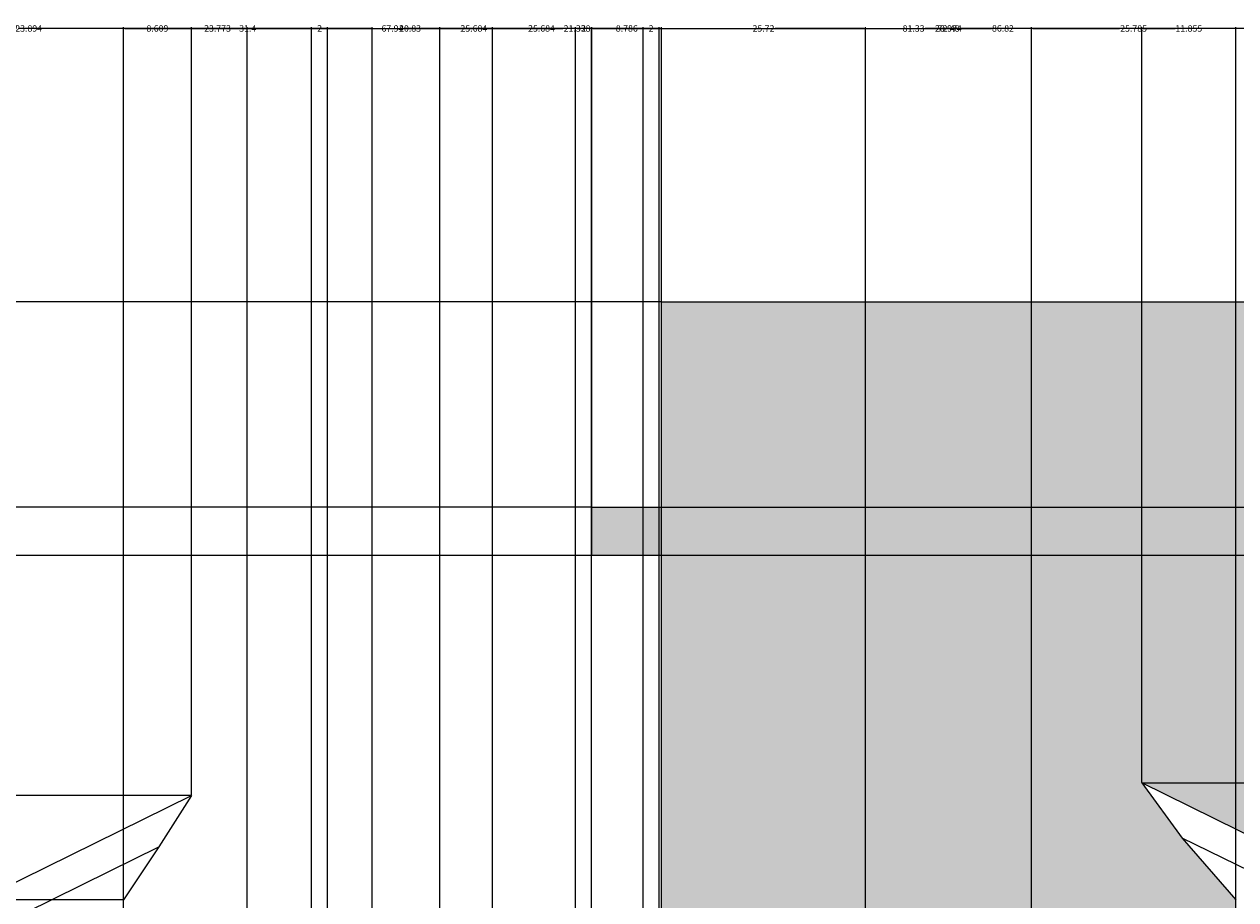
# Model space of a CAD drawing. Units: inches. Extents: x 36 to 594, y 79 to 831.
# Tile 24 of 30: x 189 to 342, y 721 to 831. Entities that reach past the tile are written whole.
import ezdxf

# ---------------------------------------------------------------- set-up
doc = ezdxf.new("R2010")
doc.units = ezdxf.units.IN
doc.header["$MEASUREMENT"] = 0
for name, color, linetype, lineweight in [('A-ANNO-DIMS', 2, 'Continuous', 18), ('A-ELEV', 7, 'Continuous', 25), ('A-ELEV-PATT', 8, 'Continuous', 13)]:
    doc.layers.add(name, color=color, linetype=linetype, lineweight=lineweight)
doc.styles.get("Standard").update_dxf_attribs({"font": 'arial.ttf'})
doc.dimstyles.get("Standard").update_dxf_attribs({"dimtxt": 0.8125, "dimasz": 0.18, "dimexe": 0.18, "dimexo": 0.0625, "dimgap": 0.09, "dimtad": 0, "dimtih": 1, "dimtoh": 1, "dimdec": 4, "dimzin": 0, "dimdsep": 46, "dimlunit": 4, "dimtxsty": 'Standard', "dimcen": 0.09, "dimadec": 0, "dimazin": 0, "dimtfac": 1, "dimtdec": 4, "dimtofl": 0, "dimtmove": 0, "dimatfit": 3, "dimfxl": 1, "dimtolj": 1, "dimtzin": 0, "dimarcsym": 0})

# ---------------------------------------------------------------- blocks, each defined once
blk = doc.blocks.new('*D14')
at = {"layer": 'A-ANNO-DIMS', "color": 0, "lineweight": -2, "transparency": 16777216}
for p, q in [((177.52, 594.27), (177.52, 830.73)), ((177.7, 830.55), (187.69, 830.55)), ((201.24, 830.55), (191.25, 830.55)), ((201.42, 720.66), (201.42, 830.73))]:
    blk.add_line(p, q, dxfattribs=at)
at = {"layer": 'A-ANNO-DIMS', "color": 0, "transparency": 16777216}
for points in [[(177.7, 830.58), (177.7, 830.52), (177.52, 830.55)], [(201.24, 830.58), (201.24, 830.52), (201.42, 830.55)]]:
    blk.add_solid(points, dxfattribs=at)
at = {"layer": 'Defpoints', "color": 0, "transparency": 16777216}
for p in [(201.42, 830.55), (201.42, 720.59), (177.52, 594.21)]:
    blk.add_point(p, dxfattribs=at)
at = {"layer": 'A-ANNO-DIMS', "color": 0, "transparency": 16777216, "insert": (189.47, 830.55), "char_height": 0.812, "attachment_point": 5}
blk.add_mtext('\\A1;23.894', dxfattribs=at)
blk = doc.blocks.new('*D15')
at = {"layer": 'A-ANNO-DIMS', "color": 0, "lineweight": -2, "transparency": 16777216}
for p, q in [((201.42, 720.66), (201.42, 830.73)), ((201.6, 830.55), (233.93, 830.55)), ((269.18, 830.55), (236.85, 830.55)), ((269.36, 796.11), (269.36, 830.73))]:
    blk.add_line(p, q, dxfattribs=at)
at = {"layer": 'A-ANNO-DIMS', "color": 0, "transparency": 16777216}
for points in [[(201.6, 830.58), (201.6, 830.52), (201.42, 830.55)], [(269.18, 830.58), (269.18, 830.52), (269.36, 830.55)]]:
    blk.add_solid(points, dxfattribs=at)
at = {"layer": 'Defpoints', "color": 0, "transparency": 16777216}
for p in [(269.36, 830.55), (269.36, 796.05), (201.42, 720.59)]:
    blk.add_point(p, dxfattribs=at)
at = {"layer": 'A-ANNO-DIMS', "color": 0, "transparency": 16777216, "insert": (235.39, 830.55), "char_height": 0.812, "attachment_point": 5}
blk.add_mtext('\\A1;67.94', dxfattribs=at)
blk = doc.blocks.new('*D16')
at = {"layer": 'A-ANNO-DIMS', "color": 0, "lineweight": -2, "transparency": 16777216}
for p, q in [((269.36, 796.11), (269.36, 830.73)), ((269.54, 830.55), (304.14, 830.55)), ((341.66, 830.55), (307.06, 830.55)), ((341.84, 720.66), (341.84, 830.73))]:
    blk.add_line(p, q, dxfattribs=at)
at = {"layer": 'A-ANNO-DIMS', "color": 0, "transparency": 16777216}
for points in [[(269.54, 830.58), (269.54, 830.52), (269.36, 830.55)], [(341.66, 830.58), (341.66, 830.52), (341.84, 830.55)]]:
    blk.add_solid(points, dxfattribs=at)
at = {"layer": 'Defpoints', "color": 0, "transparency": 16777216}
for p in [(341.84, 830.55), (269.36, 796.05), (341.84, 720.59)]:
    blk.add_point(p, dxfattribs=at)
at = {"layer": 'A-ANNO-DIMS', "color": 0, "transparency": 16777216, "insert": (305.6, 830.55), "char_height": 0.812, "attachment_point": 5}
blk.add_mtext('\\A1;72.48', dxfattribs=at)
blk = doc.blocks.new('*D22')
at = {"layer": 'A-ANNO-DIMS', "color": 0, "lineweight": -2, "transparency": 16777216}
for p, q in [((201.42, 720.66), (201.42, 830.73)), ((201.6, 830.55), (204.26, 830.55)), ((209.85, 830.55), (207.19, 830.55)), ((210.03, 733.8), (210.03, 830.73))]:
    blk.add_line(p, q, dxfattribs=at)
at = {"layer": 'A-ANNO-DIMS', "color": 0, "transparency": 16777216}
for points in [[(201.6, 830.58), (201.6, 830.52), (201.42, 830.55)], [(209.85, 830.58), (209.85, 830.52), (210.03, 830.55)]]:
    blk.add_solid(points, dxfattribs=at)
at = {"layer": 'Defpoints', "color": 0, "transparency": 16777216}
for p in [(210.03, 830.55), (210.03, 733.74), (201.42, 720.59)]:
    blk.add_point(p, dxfattribs=at)
at = {"layer": 'A-ANNO-DIMS', "color": 0, "transparency": 16777216, "insert": (205.72, 830.55), "char_height": 0.812, "attachment_point": 5}
blk.add_mtext('\\A1;8.609', dxfattribs=at)
blk = doc.blocks.new('*D23')
at = {"layer": 'A-ANNO-DIMS', "color": 0, "lineweight": -2, "transparency": 16777216}
for p, q in [((329.98, 735.4), (329.98, 830.73)), ((330.16, 830.55), (334.17, 830.55)), ((341.66, 830.55), (337.65, 830.55)), ((341.84, 720.66), (341.84, 830.73))]:
    blk.add_line(p, q, dxfattribs=at)
at = {"layer": 'A-ANNO-DIMS', "color": 0, "transparency": 16777216}
for points in [[(330.16, 830.58), (330.16, 830.52), (329.98, 830.55)], [(341.66, 830.58), (341.66, 830.52), (341.84, 830.55)]]:
    blk.add_solid(points, dxfattribs=at)
at = {"layer": 'Defpoints', "color": 0, "transparency": 16777216}
for p in [(341.84, 830.55), (329.98, 735.34), (341.84, 720.59)]:
    blk.add_point(p, dxfattribs=at)
at = {"layer": 'A-ANNO-DIMS', "color": 0, "transparency": 16777216, "insert": (335.91, 830.55), "char_height": 0.812, "attachment_point": 5}
blk.add_mtext('\\A1;11.855', dxfattribs=at)
blk = doc.blocks.new('*D25')
at = {"layer": 'A-ANNO-DIMS', "color": 0, "lineweight": -2, "transparency": 16777216}
for p, q in [((260.57, 764.1), (260.57, 830.73)), ((260.75, 830.55), (263.5, 830.55)), ((269.18, 830.55), (266.43, 830.55)), ((269.36, 796.11), (269.36, 830.73))]:
    blk.add_line(p, q, dxfattribs=at)
at = {"layer": 'A-ANNO-DIMS', "color": 0, "transparency": 16777216}
for points in [[(260.75, 830.58), (260.75, 830.52), (260.57, 830.55)], [(269.18, 830.58), (269.18, 830.52), (269.36, 830.55)]]:
    blk.add_solid(points, dxfattribs=at)
at = {"layer": 'Defpoints', "color": 0, "transparency": 16777216}
for p in [(269.36, 830.55), (269.36, 796.05), (260.57, 764.03)]:
    blk.add_point(p, dxfattribs=at)
at = {"layer": 'A-ANNO-DIMS', "color": 0, "transparency": 16777216, "insert": (264.97, 830.55), "char_height": 0.812, "attachment_point": 5}
blk.add_mtext('\\A1;8.786', dxfattribs=at)
blk = doc.blocks.new('*D28')
at = {"layer": 'A-ANNO-DIMS', "color": 0, "lineweight": -2, "transparency": 16777216}
for p, q in [((269.3, 796.05), (37.49, 796.05)), ((37.67, 795.87), (37.67, 455.63)), ((37.67, 114.39), (37.67, 454.62)), ((94.8, 114.21), (37.49, 114.21))]:
    blk.add_line(p, q, dxfattribs=at)
at = {"layer": 'A-ANNO-DIMS', "color": 0, "transparency": 16777216}
for points in [[(37.64, 795.87), (37.7, 795.87), (37.67, 796.05)], [(37.64, 114.39), (37.7, 114.39), (37.67, 114.21)]]:
    blk.add_solid(points, dxfattribs=at)
at = {"layer": 'Defpoints', "color": 0, "transparency": 16777216}
for p in [(37.67, 796.05), (269.36, 796.05), (94.87, 114.21)]:
    blk.add_point(p, dxfattribs=at)
at = {"layer": 'A-ANNO-DIMS', "color": 0, "transparency": 16777216, "insert": (37.67, 455.13), "char_height": 0.812, "attachment_point": 5}
blk.add_mtext('\\A1;681.8', dxfattribs=at)
blk = doc.blocks.new('*D37')
at = {"layer": 'A-ANNO-DIMS', "color": 0, "lineweight": -2, "transparency": 16777216}
for p, q in [((330.04, 735.34), (592.85, 735.34)), ((592.67, 735.16), (592.67, 702.28)), ((592.67, 668.39), (592.67, 701.27)), ((448.45, 668.21), (592.85, 668.21))]:
    blk.add_line(p, q, dxfattribs=at)
at = {"layer": 'A-ANNO-DIMS', "color": 0, "transparency": 16777216}
for points in [[(592.64, 735.16), (592.7, 735.16), (592.67, 735.34)], [(592.64, 668.39), (592.7, 668.39), (592.67, 668.21)]]:
    blk.add_solid(points, dxfattribs=at)
at = {"layer": 'Defpoints', "color": 0, "transparency": 16777216}
for p in [(329.98, 735.34), (592.67, 735.34), (448.39, 668.21)]:
    blk.add_point(p, dxfattribs=at)
at = {"layer": 'A-ANNO-DIMS', "color": 0, "transparency": 16777216, "insert": (592.67, 701.77), "char_height": 0.812, "attachment_point": 5}
blk.add_mtext('\\A1;67.12', dxfattribs=at)
blk = doc.blocks.new('*D38')
at = {"layer": 'A-ANNO-DIMS', "color": 0, "lineweight": -2, "transparency": 16777216}
for p, q in [((398.15, 796.05), (592.85, 796.05)), ((592.67, 795.87), (592.67, 766.2)), ((592.67, 735.52), (592.67, 765.19)), ((330.04, 735.34), (592.85, 735.34))]:
    blk.add_line(p, q, dxfattribs=at)
at = {"layer": 'A-ANNO-DIMS', "color": 0, "transparency": 16777216}
for points in [[(592.64, 795.87), (592.7, 795.87), (592.67, 796.05)], [(592.64, 735.52), (592.7, 735.52), (592.67, 735.34)]]:
    blk.add_solid(points, dxfattribs=at)
at = {"layer": 'Defpoints', "color": 0, "transparency": 16777216}
for p in [(398.09, 796.05), (592.67, 796.05), (329.98, 735.34)]:
    blk.add_point(p, dxfattribs=at)
at = {"layer": 'A-ANNO-DIMS', "color": 0, "transparency": 16777216, "insert": (592.67, 765.69), "char_height": 0.812, "attachment_point": 5}
blk.add_mtext('\\A1;60.71', dxfattribs=at)
blk = doc.blocks.new('*D48')
at = {"layer": 'A-ANNO-DIMS', "color": 0, "lineweight": -2, "transparency": 16777216}
for p, q in [((201.36, 720.59), (37.49, 720.59)), ((37.67, 720.41), (37.67, 694.91)), ((37.67, 668.39), (37.67, 693.9)), ((94.8, 668.21), (37.49, 668.21))]:
    blk.add_line(p, q, dxfattribs=at)
at = {"layer": 'A-ANNO-DIMS', "color": 0, "transparency": 16777216}
for points in [[(37.64, 720.41), (37.7, 720.41), (37.67, 720.59)], [(37.64, 668.39), (37.7, 668.39), (37.67, 668.21)]]:
    blk.add_solid(points, dxfattribs=at)
at = {"layer": 'Defpoints', "color": 0, "transparency": 16777216}
for p in [(37.67, 720.59), (201.42, 720.59), (94.87, 668.21)]:
    blk.add_point(p, dxfattribs=at)
at = {"layer": 'A-ANNO-DIMS', "color": 0, "transparency": 16777216, "insert": (37.67, 694.4), "char_height": 0.812, "attachment_point": 5}
blk.add_mtext('\\A1;52.38', dxfattribs=at)
blk = doc.blocks.new('*D49')
at = {"layer": 'A-ANNO-DIMS', "color": 0, "lineweight": -2, "transparency": 16777216}
for p, q in [((209.97, 733.74), (37.49, 733.74)), ((37.67, 733.56), (37.67, 727.67)), ((37.67, 720.77), (37.67, 726.66)), ((201.36, 720.59), (37.49, 720.59))]:
    blk.add_line(p, q, dxfattribs=at)
at = {"layer": 'A-ANNO-DIMS', "color": 0, "transparency": 16777216}
for points in [[(37.64, 733.56), (37.7, 733.56), (37.67, 733.74)], [(37.64, 720.77), (37.7, 720.77), (37.67, 720.59)]]:
    blk.add_solid(points, dxfattribs=at)
at = {"layer": 'Defpoints', "color": 0, "transparency": 16777216}
for p in [(37.67, 733.74), (210.03, 733.74), (201.42, 720.59)]:
    blk.add_point(p, dxfattribs=at)
at = {"layer": 'A-ANNO-DIMS', "color": 0, "transparency": 16777216, "insert": (37.67, 727.17), "char_height": 0.812, "attachment_point": 5}
blk.add_mtext('\\A1;13.147', dxfattribs=at)
blk = doc.blocks.new('*D50')
at = {"layer": 'A-ANNO-DIMS', "color": 0, "lineweight": -2, "transparency": 16777216}
for p, q in [((260.51, 764.03), (37.49, 764.03)), ((37.67, 763.85), (37.67, 749.39)), ((37.67, 733.92), (37.67, 748.38)), ((209.97, 733.74), (37.49, 733.74))]:
    blk.add_line(p, q, dxfattribs=at)
at = {"layer": 'A-ANNO-DIMS', "color": 0, "transparency": 16777216}
for points in [[(37.64, 763.85), (37.7, 763.85), (37.67, 764.03)], [(37.64, 733.92), (37.7, 733.92), (37.67, 733.74)]]:
    blk.add_solid(points, dxfattribs=at)
at = {"layer": 'Defpoints', "color": 0, "transparency": 16777216}
for p in [(37.67, 764.03), (260.57, 764.03), (210.03, 733.74)]:
    blk.add_point(p, dxfattribs=at)
at = {"layer": 'A-ANNO-DIMS', "color": 0, "transparency": 16777216, "insert": (37.67, 748.89), "char_height": 0.812, "attachment_point": 5}
blk.add_mtext('\\A1;30.29', dxfattribs=at)
blk = doc.blocks.new('*D51')
at = {"layer": 'A-ANNO-DIMS', "color": 0, "lineweight": -2, "transparency": 16777216}
for p, q in [((260.51, 770.15), (37.49, 770.15)), ((37.67, 769.97), (37.67, 767.59)), ((37.67, 764.21), (37.67, 766.58)), ((260.51, 764.03), (37.49, 764.03))]:
    blk.add_line(p, q, dxfattribs=at)
at = {"layer": 'A-ANNO-DIMS', "color": 0, "transparency": 16777216}
for points in [[(37.64, 769.97), (37.7, 769.97), (37.67, 770.15)], [(37.64, 764.21), (37.7, 764.21), (37.67, 764.03)]]:
    blk.add_solid(points, dxfattribs=at)
at = {"layer": 'Defpoints', "color": 0, "transparency": 16777216}
for p in [(37.67, 770.15), (260.57, 770.15), (260.57, 764.03)]:
    blk.add_point(p, dxfattribs=at)
at = {"layer": 'A-ANNO-DIMS', "color": 0, "transparency": 16777216, "insert": (37.67, 767.09), "char_height": 0.812, "attachment_point": 5}
blk.add_mtext('\\A1;6.111', dxfattribs=at)
blk = doc.blocks.new('*D52')
at = {"layer": 'A-ANNO-DIMS', "color": 0, "lineweight": -2, "transparency": 16777216}
for p, q in [((269.3, 796.05), (37.49, 796.05)), ((37.67, 795.87), (37.67, 783.6)), ((37.67, 770.33), (37.67, 782.59)), ((260.51, 770.15), (37.49, 770.15))]:
    blk.add_line(p, q, dxfattribs=at)
at = {"layer": 'A-ANNO-DIMS', "color": 0, "transparency": 16777216}
for points in [[(37.64, 795.87), (37.7, 795.87), (37.67, 796.05)], [(37.64, 770.33), (37.7, 770.33), (37.67, 770.15)]]:
    blk.add_solid(points, dxfattribs=at)
at = {"layer": 'Defpoints', "color": 0, "transparency": 16777216}
for p in [(37.67, 796.05), (269.36, 796.05), (260.57, 770.15)]:
    blk.add_point(p, dxfattribs=at)
at = {"layer": 'A-ANNO-DIMS', "color": 0, "transparency": 16777216, "insert": (37.67, 783.1), "char_height": 0.812, "attachment_point": 5}
blk.add_mtext('\\A1;25.9', dxfattribs=at)
blk = doc.blocks.new('*D61')
at = {"layer": 'A-ANNO-DIMS', "color": 0, "lineweight": -2, "transparency": 16777216}
for p, q in [((156.41, 264.68), (156.41, 830.73)), ((156.59, 830.55), (185.26, 830.55)), ((216.85, 830.55), (188.18, 830.55)), ((217.03, 286.24), (217.03, 830.73))]:
    blk.add_line(p, q, dxfattribs=at)
at = {"layer": 'A-ANNO-DIMS', "color": 0, "transparency": 16777216}
for points in [[(156.59, 830.58), (156.59, 830.52), (156.41, 830.55)], [(216.85, 830.58), (216.85, 830.52), (217.03, 830.55)]]:
    blk.add_solid(points, dxfattribs=at)
at = {"layer": 'Defpoints', "color": 0, "transparency": 16777216}
for p in [(217.03, 830.55), (217.03, 286.18), (156.41, 264.62)]:
    blk.add_point(p, dxfattribs=at)
at = {"layer": 'A-ANNO-DIMS', "color": 0, "transparency": 16777216, "insert": (186.72, 830.55), "char_height": 0.812, "attachment_point": 5}
blk.add_mtext('\\A1;60.62', dxfattribs=at)
blk = doc.blocks.new('*D92')
at = {"layer": 'A-ANNO-DIMS', "color": 0, "lineweight": -2, "transparency": 16777216}
for p, q in [((201.42, 475.48), (201.42, 830.73)), ((201.6, 830.55), (215.98, 830.55)), ((232.64, 830.55), (218.26, 830.55)), ((232.82, 524.67), (232.82, 830.73))]:
    blk.add_line(p, q, dxfattribs=at)
at = {"layer": 'A-ANNO-DIMS', "color": 0, "transparency": 16777216}
for points in [[(201.6, 830.58), (201.6, 830.52), (201.42, 830.55)], [(232.64, 830.58), (232.64, 830.52), (232.82, 830.55)]]:
    blk.add_solid(points, dxfattribs=at)
at = {"layer": 'Defpoints', "color": 0, "transparency": 16777216}
for p in [(232.82, 830.55), (232.82, 524.6), (201.42, 475.41)]:
    blk.add_point(p, dxfattribs=at)
at = {"layer": 'A-ANNO-DIMS', "color": 0, "transparency": 16777216, "insert": (217.12, 830.55), "char_height": 0.812, "attachment_point": 5}
blk.add_mtext('\\A1;31.4', dxfattribs=at)
blk = doc.blocks.new('*D93')
at = {"layer": 'A-ANNO-DIMS', "color": 0, "lineweight": -2, "transparency": 16777216}
for p, q in [((232.82, 524.67), (232.82, 830.73)), ((233, 830.55), (243.88, 830.55)), ((258.33, 830.55), (247.45, 830.55)), ((258.51, 524.67), (258.51, 830.73))]:
    blk.add_line(p, q, dxfattribs=at)
at = {"layer": 'A-ANNO-DIMS', "color": 0, "transparency": 16777216}
for points in [[(233, 830.58), (233, 830.52), (232.82, 830.55)], [(258.33, 830.58), (258.33, 830.52), (258.51, 830.55)]]:
    blk.add_solid(points, dxfattribs=at)
at = {"layer": 'Defpoints', "color": 0, "transparency": 16777216}
for p in [(258.51, 830.55), (232.82, 524.6), (258.51, 524.6)]:
    blk.add_point(p, dxfattribs=at)
at = {"layer": 'A-ANNO-DIMS', "color": 0, "transparency": 16777216, "insert": (245.66, 830.55), "char_height": 0.812, "attachment_point": 5}
blk.add_mtext('\\A1;25.684', dxfattribs=at)
blk = doc.blocks.new('*D94')
at = {"layer": 'A-ANNO-DIMS', "color": 0, "lineweight": -2, "transparency": 16777216}
for p, q in [((258.51, 524.67), (258.51, 830.73)), ((258.69, 830.55), (259.15, 830.55)), ((260.33, 830.55), (259.86, 830.55)), ((260.51, 524.67), (260.51, 830.73))]:
    blk.add_line(p, q, dxfattribs=at)
at = {"layer": 'A-ANNO-DIMS', "color": 0, "transparency": 16777216}
for points in [[(258.69, 830.58), (258.69, 830.52), (258.51, 830.55)], [(260.33, 830.58), (260.33, 830.52), (260.51, 830.55)]]:
    blk.add_solid(points, dxfattribs=at)
at = {"layer": 'Defpoints', "color": 0, "transparency": 16777216}
for p in [(260.51, 830.55), (258.51, 524.6), (260.51, 524.6)]:
    blk.add_point(p, dxfattribs=at)
at = {"layer": 'A-ANNO-DIMS', "color": 0, "transparency": 16777216, "insert": (259.51, 830.55), "char_height": 0.812, "attachment_point": 5}
blk.add_mtext('\\A1;2', dxfattribs=at)
blk = doc.blocks.new('*D95')
at = {"layer": 'A-ANNO-DIMS', "color": 0, "lineweight": -2, "transparency": 16777216}
for p, q in [((260.51, 524.67), (260.51, 830.73)), ((260.69, 830.55), (299.71, 830.55)), ((341.66, 830.55), (302.63, 830.55)), ((341.84, 524.67), (341.84, 830.73))]:
    blk.add_line(p, q, dxfattribs=at)
at = {"layer": 'A-ANNO-DIMS', "color": 0, "transparency": 16777216}
for points in [[(260.69, 830.58), (260.69, 830.52), (260.51, 830.55)], [(341.66, 830.58), (341.66, 830.52), (341.84, 830.55)]]:
    blk.add_solid(points, dxfattribs=at)
at = {"layer": 'Defpoints', "color": 0, "transparency": 16777216}
for p in [(341.84, 830.55), (260.51, 524.6), (341.84, 524.6)]:
    blk.add_point(p, dxfattribs=at)
at = {"layer": 'A-ANNO-DIMS', "color": 0, "transparency": 16777216, "insert": (301.17, 830.55), "char_height": 0.812, "attachment_point": 5}
blk.add_mtext('\\A1;81.33', dxfattribs=at)
blk = doc.blocks.new('*D105')
at = {"layer": 'A-ANNO-DIMS', "color": 0, "lineweight": -2, "transparency": 16777216}
for p, q in [((241.36, 404.34), (241.36, 830.73)), ((241.54, 830.55), (252.42, 830.55)), ((266.86, 830.55), (255.98, 830.55)), ((267.04, 404.34), (267.04, 830.73))]:
    blk.add_line(p, q, dxfattribs=at)
at = {"layer": 'A-ANNO-DIMS', "color": 0, "transparency": 16777216}
for points in [[(241.54, 830.58), (241.54, 830.52), (241.36, 830.55)], [(266.86, 830.58), (266.86, 830.52), (267.04, 830.55)]]:
    blk.add_solid(points, dxfattribs=at)
at = {"layer": 'Defpoints', "color": 0, "transparency": 16777216}
for p in [(267.04, 830.55), (241.36, 404.27), (267.04, 404.27)]:
    blk.add_point(p, dxfattribs=at)
at = {"layer": 'A-ANNO-DIMS', "color": 0, "transparency": 16777216, "insert": (254.2, 830.55), "char_height": 0.812, "attachment_point": 5}
blk.add_mtext('\\A1;25.684', dxfattribs=at)
blk = doc.blocks.new('*D106')
at = {"layer": 'A-ANNO-DIMS', "color": 0, "lineweight": -2, "transparency": 16777216}
for p, q in [((267.04, 404.34), (267.04, 830.73)), ((267.22, 830.55), (267.68, 830.55)), ((268.86, 830.55), (268.4, 830.55)), ((269.04, 404.34), (269.04, 830.73))]:
    blk.add_line(p, q, dxfattribs=at)
at = {"layer": 'A-ANNO-DIMS', "color": 0, "transparency": 16777216}
for points in [[(267.22, 830.58), (267.22, 830.52), (267.04, 830.55)], [(268.86, 830.58), (268.86, 830.52), (269.04, 830.55)]]:
    blk.add_solid(points, dxfattribs=at)
at = {"layer": 'Defpoints', "color": 0, "transparency": 16777216}
for p in [(269.04, 830.55), (267.04, 404.27), (269.04, 404.27)]:
    blk.add_point(p, dxfattribs=at)
at = {"layer": 'A-ANNO-DIMS', "color": 0, "transparency": 16777216, "insert": (268.04, 830.55), "char_height": 0.812, "attachment_point": 5}
blk.add_mtext('\\A1;2', dxfattribs=at)
blk = doc.blocks.new('*D107')
at = {"layer": 'A-ANNO-DIMS', "color": 0, "lineweight": -2, "transparency": 16777216}
for p, q in [((269.04, 404.34), (269.04, 830.73)), ((269.22, 830.55), (310.99, 830.55)), ((355.68, 830.55), (313.91, 830.55)), ((355.86, 404.34), (355.86, 830.73))]:
    blk.add_line(p, q, dxfattribs=at)
at = {"layer": 'A-ANNO-DIMS', "color": 0, "transparency": 16777216}
for points in [[(269.22, 830.58), (269.22, 830.52), (269.04, 830.55)], [(355.68, 830.58), (355.68, 830.52), (355.86, 830.55)]]:
    blk.add_solid(points, dxfattribs=at)
at = {"layer": 'Defpoints', "color": 0, "transparency": 16777216}
for p in [(355.86, 830.55), (269.04, 404.27), (355.86, 404.27)]:
    blk.add_point(p, dxfattribs=at)
at = {"layer": 'A-ANNO-DIMS', "color": 0, "transparency": 16777216, "insert": (312.45, 830.55), "char_height": 0.812, "attachment_point": 5}
blk.add_mtext('\\A1;86.82', dxfattribs=at)
blk = doc.blocks.new('*D123')
at = {"layer": 'A-ANNO-DIMS', "color": 0, "lineweight": -2, "transparency": 16777216}
for p, q in [((201.42, 630.1), (201.42, 830.73)), ((201.6, 830.55), (211.52, 830.55)), ((225.01, 830.55), (215.09, 830.55)), ((225.19, 630.1), (225.19, 830.73))]:
    blk.add_line(p, q, dxfattribs=at)
at = {"layer": 'A-ANNO-DIMS', "color": 0, "transparency": 16777216}
for points in [[(201.6, 830.58), (201.6, 830.52), (201.42, 830.55)], [(225.01, 830.58), (225.01, 830.52), (225.19, 830.55)]]:
    blk.add_solid(points, dxfattribs=at)
at = {"layer": 'Defpoints', "color": 0, "transparency": 16777216}
for p in [(225.19, 830.55), (201.42, 630.04), (225.19, 630.04)]:
    blk.add_point(p, dxfattribs=at)
at = {"layer": 'A-ANNO-DIMS', "color": 0, "transparency": 16777216, "insert": (213.31, 830.55), "char_height": 0.812, "attachment_point": 5}
blk.add_mtext('\\A1;23.773', dxfattribs=at)
blk = doc.blocks.new('*D124')
at = {"layer": 'A-ANNO-DIMS', "color": 0, "lineweight": -2, "transparency": 16777216}
for p, q in [((225.19, 630.1), (225.19, 830.73)), ((225.37, 830.55), (225.83, 830.55)), ((227.01, 830.55), (226.55, 830.55)), ((227.19, 630.1), (227.19, 830.73))]:
    blk.add_line(p, q, dxfattribs=at)
at = {"layer": 'A-ANNO-DIMS', "color": 0, "transparency": 16777216}
for points in [[(225.37, 830.58), (225.37, 830.52), (225.19, 830.55)], [(227.01, 830.58), (227.01, 830.52), (227.19, 830.55)]]:
    blk.add_solid(points, dxfattribs=at)
at = {"layer": 'Defpoints', "color": 0, "transparency": 16777216}
for p in [(227.19, 830.55), (225.19, 630.04), (227.19, 630.04)]:
    blk.add_point(p, dxfattribs=at)
at = {"layer": 'A-ANNO-DIMS', "color": 0, "transparency": 16777216, "insert": (226.19, 830.55), "char_height": 0.812, "attachment_point": 5}
blk.add_mtext('\\A1;2', dxfattribs=at)
blk = doc.blocks.new('*D125')
at = {"layer": 'A-ANNO-DIMS', "color": 0, "lineweight": -2, "transparency": 16777216}
for p, q in [((227.19, 630.1), (227.19, 830.73)), ((227.37, 830.55), (236.14, 830.55)), ((247.84, 830.55), (239.07, 830.55)), ((248.02, 630.27), (248.02, 830.73))]:
    blk.add_line(p, q, dxfattribs=at)
at = {"layer": 'A-ANNO-DIMS', "color": 0, "transparency": 16777216}
for points in [[(227.37, 830.58), (227.37, 830.52), (227.19, 830.55)], [(247.84, 830.58), (247.84, 830.52), (248.02, 830.55)]]:
    blk.add_solid(points, dxfattribs=at)
at = {"layer": 'Defpoints', "color": 0, "transparency": 16777216}
for p in [(248.02, 830.55), (248.02, 630.21), (227.19, 630.04)]:
    blk.add_point(p, dxfattribs=at)
at = {"layer": 'A-ANNO-DIMS', "color": 0, "transparency": 16777216, "insert": (237.61, 830.55), "char_height": 0.812, "attachment_point": 5}
blk.add_mtext('\\A1;20.83', dxfattribs=at)
blk = doc.blocks.new('*D126')
at = {"layer": 'A-ANNO-DIMS', "color": 0, "lineweight": -2, "transparency": 16777216}
for p, q in [((248.02, 630.27), (248.02, 830.73)), ((248.2, 830.55), (256.91, 830.55)), ((269.18, 830.55), (260.47, 830.55)), ((269.36, 630.1), (269.36, 830.73))]:
    blk.add_line(p, q, dxfattribs=at)
at = {"layer": 'A-ANNO-DIMS', "color": 0, "transparency": 16777216}
for points in [[(248.2, 830.58), (248.2, 830.52), (248.02, 830.55)], [(269.18, 830.58), (269.18, 830.52), (269.36, 830.55)]]:
    blk.add_solid(points, dxfattribs=at)
at = {"layer": 'Defpoints', "color": 0, "transparency": 16777216}
for p in [(269.36, 830.55), (248.02, 630.21), (269.36, 630.04)]:
    blk.add_point(p, dxfattribs=at)
at = {"layer": 'A-ANNO-DIMS', "color": 0, "transparency": 16777216, "insert": (258.69, 830.55), "char_height": 0.812, "attachment_point": 5}
blk.add_mtext('\\A1;21.338', dxfattribs=at)
blk = doc.blocks.new('*D127')
at = {"layer": 'A-ANNO-DIMS', "color": 0, "lineweight": -2, "transparency": 16777216}
for p, q in [((269.36, 630.1), (269.36, 830.73)), ((269.54, 830.55), (280.75, 830.55)), ((294.9, 830.55), (283.68, 830.55)), ((295.08, 630.1), (295.08, 830.73))]:
    blk.add_line(p, q, dxfattribs=at)
at = {"layer": 'A-ANNO-DIMS', "color": 0, "transparency": 16777216}
for points in [[(269.54, 830.58), (269.54, 830.52), (269.36, 830.55)], [(294.9, 830.58), (294.9, 830.52), (295.08, 830.55)]]:
    blk.add_solid(points, dxfattribs=at)
at = {"layer": 'Defpoints', "color": 0, "transparency": 16777216}
for p in [(295.08, 830.55), (269.36, 630.04), (295.08, 630.04)]:
    blk.add_point(p, dxfattribs=at)
at = {"layer": 'A-ANNO-DIMS', "color": 0, "transparency": 16777216, "insert": (282.22, 830.55), "char_height": 0.812, "attachment_point": 5}
blk.add_mtext('\\A1;25.72', dxfattribs=at)
blk = doc.blocks.new('*D128')
at = {"layer": 'A-ANNO-DIMS', "color": 0, "lineweight": -2, "transparency": 16777216}
for p, q in [((295.08, 630.1), (295.08, 830.73)), ((295.26, 830.55), (303.78, 830.55)), ((315.87, 830.55), (307.35, 830.55)), ((316.05, 630.1), (316.05, 830.73))]:
    blk.add_line(p, q, dxfattribs=at)
at = {"layer": 'A-ANNO-DIMS', "color": 0, "transparency": 16777216}
for points in [[(295.26, 830.58), (295.26, 830.52), (295.08, 830.55)], [(315.87, 830.58), (315.87, 830.52), (316.05, 830.55)]]:
    blk.add_solid(points, dxfattribs=at)
at = {"layer": 'Defpoints', "color": 0, "transparency": 16777216}
for p in [(316.05, 830.55), (295.08, 630.04), (316.05, 630.04)]:
    blk.add_point(p, dxfattribs=at)
at = {"layer": 'A-ANNO-DIMS', "color": 0, "transparency": 16777216, "insert": (305.56, 830.55), "char_height": 0.812, "attachment_point": 5}
blk.add_mtext('\\A1;20.974', dxfattribs=at)
blk = doc.blocks.new('*D129')
at = {"layer": 'A-ANNO-DIMS', "color": 0, "lineweight": -2, "transparency": 16777216}
for p, q in [((316.05, 630.1), (316.05, 830.73)), ((316.23, 830.55), (327.16, 830.55)), ((341.66, 830.55), (330.73, 830.55)), ((341.84, 630.1), (341.84, 830.73))]:
    blk.add_line(p, q, dxfattribs=at)
at = {"layer": 'A-ANNO-DIMS', "color": 0, "transparency": 16777216}
for points in [[(316.23, 830.58), (316.23, 830.52), (316.05, 830.55)], [(341.66, 830.58), (341.66, 830.52), (341.84, 830.55)]]:
    blk.add_solid(points, dxfattribs=at)
at = {"layer": 'Defpoints', "color": 0, "transparency": 16777216}
for p in [(341.84, 830.55), (316.05, 630.04), (341.84, 630.04)]:
    blk.add_point(p, dxfattribs=at)
at = {"layer": 'A-ANNO-DIMS', "color": 0, "transparency": 16777216, "insert": (328.94, 830.55), "char_height": 0.812, "attachment_point": 5}
blk.add_mtext('\\A1;25.785', dxfattribs=at)

msp = doc.modelspace()

# ---------------------------------------------------------------- hatches: boundary and pattern name
at = {"layer": 'A-ELEV-PATT'}
h = msp.add_hatch(color=256, dxfattribs=at)
h.dxf.hatch_style = 1
h.paths.add_polyline_path([(398.0873, 796.0465), (269.3592, 796.0465), (269.3592, 770.1455), (397.8159, 770.1455)])
h.paths.add_polyline_path([(397.7518, 764.0341), (269.3592, 764.0341), (269.3592, 630.0394), (341.8367, 630.0394), (341.8367, 720.595), (335.0881, 728.3699), (329.982, 735.3373), (345.3661, 727.7743), (397.1052, 702.3389)])
h.paths.add_polyline_path([(341.8367, 594.2124), (201.4189, 594.2124), (201.4189, 475.4136), (232.8216, 475.4136), (232.8216, 524.6037), (341.8367, 524.6037)])
h.paths.add_polyline_path([(177.525, 594.2124), (118.7598, 594.2124), (118.7598, 450.2124), (177.525, 450.2124)])
h.paths.add_polyline_path([(424.4958, 594.2124), (365.7306, 594.2124), (365.7306, 450.2124), (424.4958, 450.2124)])
h.paths.add_polyline_path([(241.3553, 404.2737), (355.8569, 404.2737), (355.8569, 355.0836), (424.5492, 355.0836), (424.5492, 425.7333), (118.7598, 426.2844), (118.7598, 355.0836), (241.3553, 355.0836)])
h.paths.add_polyline_path([(448.3898, 306.2124), (217.0273, 306.2124), (217.0273, 142.2124), (254.0293, 142.2124), (254.0293, 150.9347), (254.0293, 286.1802), (401.5491, 286.1802), (401.5491, 150.9347), (401.5491, 142.2124), (448.3898, 142.2124)])
h.paths.add_polyline_path([(448.3898, 142.2124), (401.5491, 142.2124), (217.0273, 142.2124), (217.0273, 114.2124), (448.3898, 114.2124)])
h.paths.add_polyline_path([(217.0273, 306.2124), (174.7353, 306.2124), (94.8658, 306.2124), (94.8658, 162.2124), (103.3368, 162.2124), (103.3368, 264.6224), (103.3368, 286.1802), (217.0273, 286.1802)])
h = msp.add_hatch(color=256, dxfattribs=at)
h.dxf.hatch_style = 1
h.paths.add_polyline_path([(94.8658, 608.6081), (72.1733, 608.6081), (72.1733, 603.598), (94.8658, 603.598)])
h.paths.add_polyline_path([(94.8658, 427.5982), (72.1733, 427.5982), (72.1733, 422.5882), (94.8658, 422.5882)])
h.paths.add_polyline_path([(94.8658, 299.486), (72.1733, 299.486), (72.1733, 294.4759), (94.8658, 294.4759)])
h.paths.add_polyline_path([(269.3592, 770.1455), (260.5727, 770.1455), (260.5727, 764.0341), (269.3592, 764.0341)])
h.paths.add_polyline_path([(410.2381, 770.1455), (269.3592, 770.1455), (269.3592, 764.0341), (410.2381, 764.0341)])

# ---------------------------------------------------------------- linework, layer by layer
at = {"layer": 'A-ELEV'}
for p, q in [((269.3592, 630.0394), (269.3592, 796.0465)), ((269.3592, 796.0465), (398.0873, 796.0465)), ((345.3661, 727.7743), (329.982, 735.3373)), ((329.982, 735.3373), (335.0881, 728.3699)), ((197.8895, 727.7743), (210.028, 733.7417)), ((210.028, 733.7417), (205.9095, 727.2598)), ((343.6014, 724.1846), (335.0881, 728.3699)), ((335.0881, 728.3699), (341.8367, 720.595)), ((91.3364, 675.3917), (197.8895, 727.7743)), ((199.6542, 724.1846), (205.9095, 727.2598)), ((205.9095, 727.2598), (201.4189, 720.595)), ((93.1011, 671.802), (199.6542, 724.1846))]:
    msp.add_line(p, q, dxfattribs=at)
msp.add_lwpolyline([(260.5727, 770.1455), (410.2381, 770.1455), (410.2381, 764.0341), (260.5727, 764.0341)], close=True, dxfattribs=at)

# ---------------------------------------------------------------- dimensions: what is measured, and where the dimension line sits
at = {"layer": 'A-ANNO-DIMS'}
for base, p1, p2, override, picture, middle in [((217.0273, 830.5465), (156.4069, 264.6224), (217.0273, 286.1802), {"dimdec": 2, "dimlfac": 1, "dimrnd": 0, "dimzin": 0, "dimdsep": 46, "dimlunit": 2}, '*D61', (186.7171, 830.5465)), ((201.4189, 830.5465), (177.525, 594.2124), (201.4189, 720.595), {"dimdec": 3, "dimlfac": 1, "dimrnd": 0, "dimzin": 0, "dimdsep": 46, "dimlunit": 2}, '*D14', (189.4719, 830.5465)), ((269.3592, 830.5465), (201.4189, 720.595), (269.3592, 796.0465), {"dimdec": 2, "dimlfac": 1, "dimrnd": 0, "dimzin": 0, "dimdsep": 46, "dimlunit": 2}, '*D15', (235.389, 830.5465)), ((210.028, 830.5465), (201.4189, 720.595), (210.028, 733.7417), {"dimdec": 3, "dimlfac": 1, "dimrnd": 0, "dimzin": 0, "dimdsep": 46, "dimlunit": 2}, '*D22', (205.7234, 830.5465)), ((232.8216, 830.5465), (201.4189, 475.4136), (232.8216, 524.6037), {"dimdec": 1, "dimlfac": 1, "dimrnd": 0, "dimzin": 0, "dimdsep": 46, "dimlunit": 2}, '*D92', (217.1202, 830.5465)), ((225.1915, 830.5465), (201.4189, 630.0394), (225.1915, 630.0394), {"dimdec": 3, "dimlfac": 1, "dimrnd": 0, "dimzin": 0, "dimdsep": 46, "dimlunit": 2}, '*D123', (213.3052, 830.5465)), ((227.1915, 830.5465), (225.1915, 630.0394), (227.1915, 630.0394), {"dimdec": 0, "dimlfac": 1, "dimrnd": 0, "dimzin": 0, "dimdsep": 46, "dimlunit": 2}, '*D124', (226.1915, 830.5465)), ((248.0217, 830.5465), (227.1915, 630.0394), (248.0217, 630.2124), {"dimdec": 2, "dimlfac": 1, "dimrnd": 0, "dimzin": 0, "dimdsep": 46, "dimlunit": 2}, '*D125', (237.6066, 830.5465)), ((258.5056, 830.5465), (232.8216, 524.6037), (258.5056, 524.6037), {"dimdec": 3, "dimlfac": 1, "dimrnd": 0, "dimzin": 0, "dimdsep": 46, "dimlunit": 2}, '*D93', (245.6636, 830.5465)), ((267.0393, 830.5465), (241.3553, 404.2737), (267.0393, 404.2737), {"dimdec": 3, "dimlfac": 1, "dimrnd": 0, "dimzin": 0, "dimdsep": 46, "dimlunit": 2}, '*D105', (254.1973, 830.5465)), ((269.35917, 830.54647), (248.02166, 630.21236), (269.35917, 630.03937), {"dimdec": 3, "dimlfac": 1, "dimrnd": 0, "dimzin": 0, "dimdsep": 46, "dimlunit": 2}, '*D126', (258.69041, 830.54647)), ((260.5056, 830.5465), (258.5056, 524.6037), (260.5056, 524.6037), {"dimdec": 0, "dimlfac": 1, "dimrnd": 0, "dimzin": 0, "dimdsep": 46, "dimlunit": 2}, '*D94', (259.5056, 830.5465)), ((341.8367, 830.5465), (260.5056, 524.6037), (341.8367, 524.6037), {"dimdec": 2, "dimlfac": 1, "dimrnd": 0, "dimzin": 0, "dimdsep": 46, "dimlunit": 2}, '*D95', (301.1711, 830.5465)), ((269.35917, 830.54647), (260.57272, 764.03414), (269.35917, 796.04647), {"dimdec": 3, "dimlfac": 1, "dimrnd": 0, "dimzin": 0, "dimdsep": 46, "dimlunit": 2}, '*D25', (264.96594, 830.54647)), ((269.0393, 830.5465), (267.0393, 404.2737), (269.0393, 404.2737), {"dimdec": 0, "dimlfac": 1, "dimrnd": 0, "dimzin": 0, "dimdsep": 46, "dimlunit": 2}, '*D106', (268.0393, 830.5465)), ((355.8569, 830.5465), (269.0393, 404.2737), (355.8569, 404.2737), {"dimdec": 2, "dimlfac": 1, "dimrnd": 0, "dimzin": 0, "dimdsep": 46, "dimlunit": 2}, '*D107', (312.4481, 830.5465)), ((341.8367, 830.5465), (269.3592, 796.0465), (341.8367, 720.595), {"dimdec": 2, "dimlfac": 1, "dimrnd": 0, "dimzin": 0, "dimdsep": 46, "dimlunit": 2}, '*D16', (305.5979, 830.5465)), ((295.0778, 830.5465), (269.3592, 630.0394), (295.0778, 630.0394), {"dimdec": 2, "dimlfac": 1, "dimrnd": 0, "dimzin": 0, "dimdsep": 46, "dimlunit": 2}, '*D127', (282.2185, 830.5465)), ((316.0513, 830.54647), (295.07777, 630.03937), (316.0513, 630.03937), {"dimdec": 3, "dimlfac": 1, "dimrnd": 0, "dimzin": 0, "dimdsep": 46, "dimlunit": 2}, '*D128', (305.56454, 830.54647)), ((341.8367, 830.5465), (316.0513, 630.0394), (341.8367, 630.0394), {"dimdec": 3, "dimlfac": 1, "dimrnd": 0, "dimzin": 0, "dimdsep": 46, "dimlunit": 2}, '*D129', (328.944, 830.5465)), ((341.8367, 830.5465), (329.982, 735.3373), (341.8367, 720.595), {"dimdec": 3, "dimlfac": 1, "dimrnd": 0, "dimzin": 0, "dimdsep": 46, "dimlunit": 2}, '*D23', (335.9093, 830.5465))]:
    dim = msp.add_linear_dim(base=base, p1=p1, p2=p2, dimstyle='Standard', override=override, dxfattribs=at)
    dim.commit()
    dim.dimension.update_dxf_attribs({"geometry": picture, "text_midpoint": middle})
for base, p1, p2, override, picture, middle in [((37.6733, 796.0465), (94.8658, 114.2124), (269.3592, 796.0465), {"dimdec": 1, "dimlfac": 1, "dimrnd": 0, "dimzin": 0, "dimdsep": 46, "dimlunit": 2}, '*D28', (37.6733, 455.1294)), ((37.6733, 796.0465), (260.5727, 770.1455), (269.3592, 796.0465), {"dimdec": 1, "dimlfac": 1, "dimrnd": 0, "dimzin": 0, "dimdsep": 46, "dimlunit": 2}, '*D52', (37.6733, 783.096)), ((592.6689, 796.0465), (329.982, 735.3373), (398.0873, 796.0465), {"dimdec": 2, "dimlfac": 1, "dimrnd": 0, "dimzin": 0, "dimdsep": 46, "dimlunit": 2}, '*D38', (592.6689, 765.6919)), ((37.6733, 770.1455), (260.5727, 764.0341), (260.5727, 770.1455), {"dimdec": 3, "dimlfac": 1, "dimrnd": 0, "dimzin": 0, "dimdsep": 46, "dimlunit": 2}, '*D51', (37.6733, 767.0898)), ((37.6733, 764.0341), (210.028, 733.7417), (260.5727, 764.0341), {"dimdec": 2, "dimlfac": 1, "dimrnd": 0, "dimzin": 0, "dimdsep": 46, "dimlunit": 2}, '*D50', (37.6733, 748.8879)), ((592.6689, 735.3373), (448.3898, 668.2124), (329.982, 735.3373), {"dimdec": 2, "dimlfac": 1, "dimrnd": 0, "dimzin": 0, "dimdsep": 46, "dimlunit": 2}, '*D37', (592.6689, 701.7748)), ((37.6733, 733.7417), (201.4189, 720.595), (210.028, 733.7417), {"dimdec": 3, "dimlfac": 1, "dimrnd": 0, "dimzin": 0, "dimdsep": 46, "dimlunit": 2}, '*D49', (37.6733, 727.1683)), ((37.6733, 720.595), (94.8658, 668.2124), (201.4189, 720.595), {"dimdec": 2, "dimlfac": 1, "dimrnd": 0, "dimzin": 0, "dimdsep": 46, "dimlunit": 2}, '*D48', (37.6733, 694.4037))]:
    dim = msp.add_linear_dim(base=base, p1=p1, p2=p2, angle=90, dimstyle='Standard', override=override, dxfattribs=at)
    dim.commit()
    dim.dimension.update_dxf_attribs({"geometry": picture, "text_midpoint": middle})

doc.saveas('drawing.dxf')
